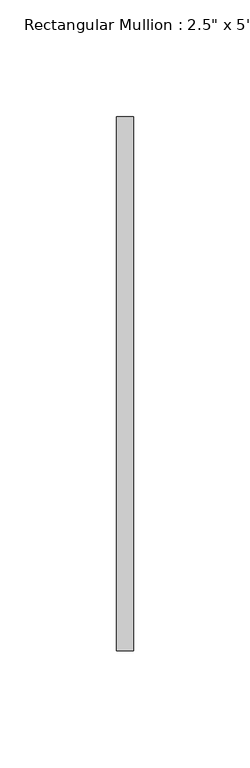
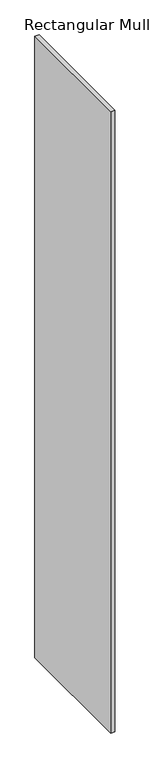
"""IFC4 building model written with IfcOpenShell, lengths in millimetres: member geometry."""

from ifc_helpers import new_model, si_unit, frame, origin, place, context, project, spatial, polyline, outline, extrude, source, transform, mapped, element, save


def member_7d5ce663(model_context):
    return source(origin(), model_context, "Body", "SweptSolid", [
        extrude(outline(polyline([(0.0, 114.3), (0.0, -114.3), (-7.239, -114.3), (-7.239, 114.3), (0.0, 114.3)])), frame((0.0, 0.0, -1144.8415), z_axis=(0.0, 0.0, 1.0), x_axis=(1.0, 0.0, 0.0)), (0.0, 0.0, 1.0), 1144.8415),
    ])


if __name__ == "__main__":
    model = new_model("IFC4")
    model_context = context("Model", 3, world=origin())
    ifc_project = project(units=[si_unit("LENGTHUNIT", "METRE", prefix="MILLI")], contexts=[model_context])
    site = spatial("IfcSite", under=ifc_project)
    building = spatial("IfcBuilding", under=site)
    placement = place(None, origin())
    member_shape = member_7d5ce663(model_context)
    element("IfcMember", 1, ObjectType="Rectangular Mullion : 2.5\" x 5\" rectangular", at=placement, inside=building, context=model_context, shape_type="MappedRepresentation", body=[
        mapped(member_shape, transform((0.0, 0.0, 0.0), x_axis=(1.0, 0.0, 0.0), y_axis=(0.0, 1.0, 0.0), z_axis=(0.0, 0.0, 1.0))),
    ])
    save(model, "model.ifc")

# Revit data of these elements
# Type "Rectangular Mullion : 2.5\" x 5\" rectangular"
#   built-in parameter 1007304 = 0.75 (stored number, unit not read)
#   built-in parameter 1007301 = 0.011875 (stored number, unit not read)
#   built-in parameter 1007300 = 0.011875 (stored number, unit not read)
# Element 1 (IfcMember, "Rectangular Mullion : 2.5\" x 5\" rectangular")
#   Materials on its faces: "WINDOW GLASS MATERIAL"
# Materials
#   "WINDOW GLASS MATERIAL": class "Generic", colour RGB 120 120 120, transparency 0, Cost = 0
